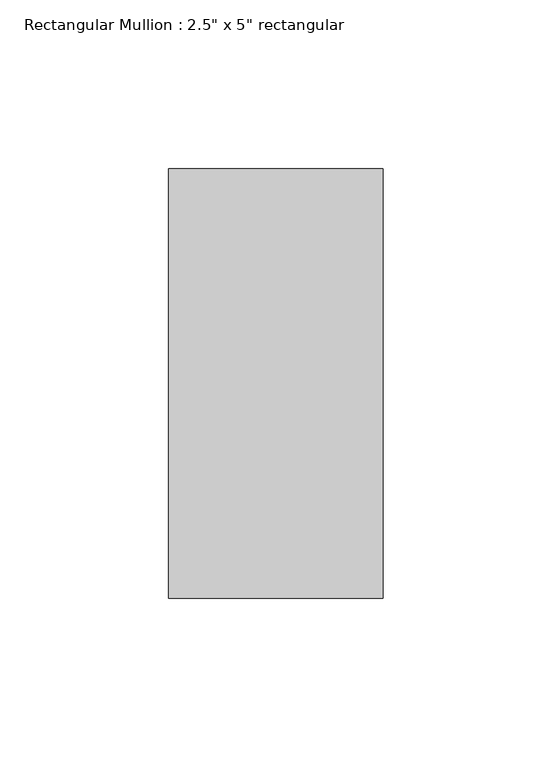
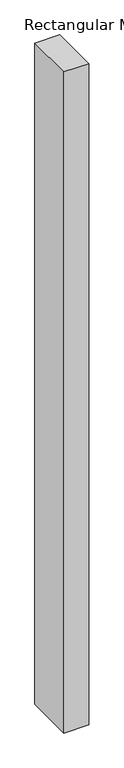
"""IFC4 building model written with IfcOpenShell, lengths in millimetres: member geometry."""

from ifc_helpers import new_model, si_unit, frame, origin, place, context, project, spatial, polyline, outline, extrude, source, transform, mapped, element, save


def member_85079546(model_context):
    return source(origin(), model_context, "Body", "SweptSolid", [
        extrude(outline(polyline([(0.0, 63.5), (0.0, -63.5), (-63.5, -63.5), (-63.5, 63.5), (0.0, 63.5)])), frame((0.0, 0.0, -1771.500021), z_axis=(0.0, 0.0, 1.0), x_axis=(1.0, 0.0, 0.0)), (0.0, 0.0, 1.0), 1771.500021),
    ])


if __name__ == "__main__":
    model = new_model("IFC4")
    model_context = context("Model", 3, world=origin())
    ifc_project = project(units=[si_unit("LENGTHUNIT", "METRE", prefix="MILLI")], contexts=[model_context])
    site = spatial("IfcSite", under=ifc_project)
    building = spatial("IfcBuilding", under=site)
    placement = place(None, origin())
    member_shape = member_85079546(model_context)
    element("IfcMember", 1, ObjectType="Rectangular Mullion : 2.5\" x 5\" rectangular", at=placement, inside=building, context=model_context, shape_type="MappedRepresentation", body=[
        mapped(member_shape, transform((0.0, 0.0, 0.0), x_axis=(1.0, 0.0, 0.0), y_axis=(0.0, 1.0, 0.0), z_axis=(0.0, 0.0, 1.0))),
    ])
    save(model, "model.ifc")

# Revit data of these elements
# Type "Rectangular Mullion : 2.5\" x 5\" rectangular"
#   built-in parameter 1007304 = 0.416667 (stored number, unit not read)
#   built-in parameter 1007301 = 0.104167 (stored number, unit not read)
#   built-in parameter 1007300 = 0.104167 (stored number, unit not read)
# Element 1 (IfcMember, "Rectangular Mullion : 2.5\" x 5\" rectangular")
#   Materials on its faces: "Aluminum"
# Materials
#   "Aluminum": class "Metal", colour RGB 247 247 247, transparency 0, Description = "Aluminum 6061", Cost = 0
